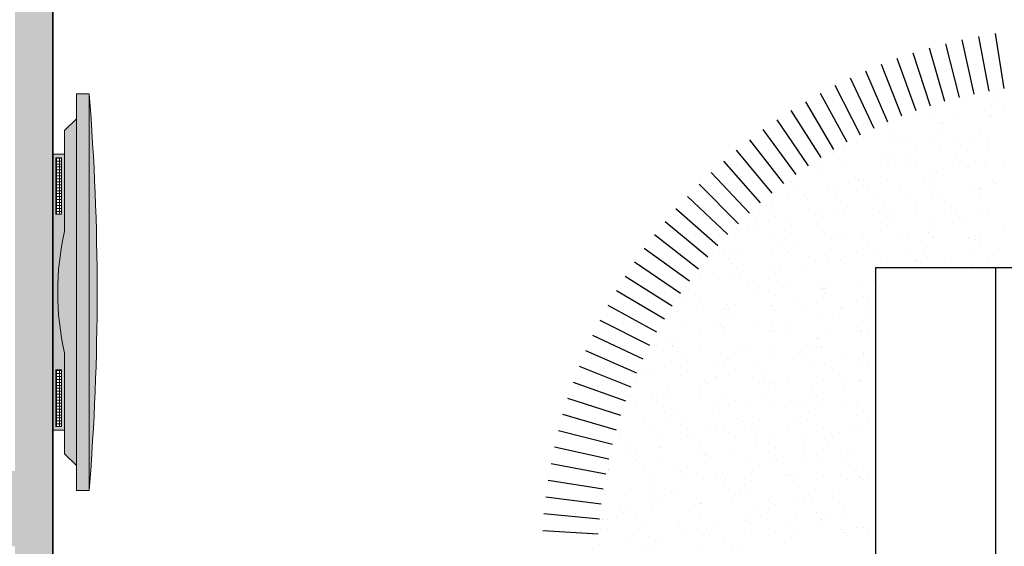
# Model space of a CAD drawing. Units: inches. Extents: x 1566 to 2546, y 1087 to 2705.
# Tile 4 of 27: x 1820 to 1925, y 1270 to 1326. Entities that reach past the tile are written whole.
import ezdxf

# ---------------------------------------------------------------- set-up
doc = ezdxf.new("R2010")
doc.units = ezdxf.units.IN
for name, color, linetype in [('A-FRN', 11, 'Continuous'), ('A-HT', 15, 'Continuous'), ('L-HT', 1, 'Continuous')]:
    doc.layers.add(name, color=color, linetype=linetype)
for name, color, linetype, lineweight in [('A-FURN', 8, 'Continuous', 18), ('A-WALL', 7, 'Continuous', 35), ('A-WALL-PATT', 8, 'Continuous', 13), ('moveis', 254, 'Continuous', 5), ('parede', 7, 'Continuous', 30)]:
    doc.layers.add(name, color=color, linetype=linetype, lineweight=lineweight)

# ---------------------------------------------------------------- blocks, each defined once
blk = doc.blocks.new('*X21')
at = {"color": 0}
for p, q in [((1.945, 2.8452), (1.945, 2.8452)), ((1.7428, 2.8186), (1.7428, 2.8186)), ((1.7438, 2.8187), (1.7438, 2.8187)), ((1.7537, 2.8227), (1.7537, 2.8227)), ((1.7698, 2.8221), (1.7698, 2.8221)), ((1.8017, 2.833), (1.8017, 2.833)), ((1.8104, 2.8275), (1.8104, 2.8275)), ((1.8778, 2.8235), (1.8778, 2.8235)), ((1.8783, 2.8364), (1.8783, 2.8364)), ((1.9044, 2.8399), (1.9044, 2.8399)), ((1.9094, 2.823), (1.9094, 2.823)), ((1.6514, 2.7891), (1.6514, 2.7891)), ((1.8515, 2.7874), (1.8515, 2.7874)), ((1.5474, 2.7675), (1.5474, 2.7675)), ((1.6825, 2.7724), (1.6825, 2.7724)), ((1.8133, 2.774), (1.8133, 2.774)), ((1.8607, 2.779), (1.8607, 2.779)), ((1.9412, 2.7734), (1.9412, 2.7734)), ((1.5011, 2.7453), (1.5011, 2.7453)), ((1.5414, 2.759), (1.5414, 2.759)), ((1.5625, 2.7456), (1.5625, 2.7456)), ((1.6971, 2.7593), (1.6971, 2.7593)), ((1.7012, 2.7435), (1.7012, 2.7435)), ((1.7104, 2.7351), (1.7104, 2.7351)), ((1.7182, 2.7459), (1.7182, 2.7459)), ((1.8528, 2.7596), (1.8528, 2.7596)), ((1.8739, 2.7462), (1.8739, 2.7462)), ((1.9042, 2.7391), (1.9042, 2.7391)), ((1.4871, 2.7212), (1.4871, 2.7212)), ((1.618, 2.7229), (1.618, 2.7229)), ((1.7459, 2.7223), (1.7459, 2.7223)), ((1.881, 2.7272), (1.881, 2.7272)), ((1.9244, 2.7131), (1.9244, 2.7131)), ((1.9505, 2.7165), (1.9505, 2.7165)), ((1.4827, 2.697), (1.4827, 2.697)), ((1.5509, 2.6997), (1.5509, 2.6997)), ((1.5601, 2.6912), (1.5601, 2.6912)), ((1.6384, 2.6973), (1.6384, 2.6973)), ((1.6813, 2.681), (1.6813, 2.681)), ((1.7219, 2.6864), (1.7219, 2.6864)), ((1.7539, 2.6952), (1.7539, 2.6952)), ((1.7899, 2.6953), (1.7899, 2.6953)), ((1.7941, 2.6975), (1.7941, 2.6975)), ((1.8159, 2.6988), (1.8159, 2.6988)), ((1.8565, 2.7041), (1.8565, 2.7041)), ((1.9498, 2.6978), (1.9498, 2.6978)), ((1.4006, 2.6558), (1.4006, 2.6558)), ((1.4227, 2.6718), (1.4227, 2.6718)), ((1.5207, 2.6599), (1.5207, 2.6599)), ((1.5467, 2.6633), (1.5467, 2.6633)), ((1.5506, 2.6712), (1.5506, 2.6712)), ((1.5873, 2.6687), (1.5873, 2.6687)), ((1.6553, 2.6776), (1.6553, 2.6776)), ((1.6856, 2.676), (1.6856, 2.676)), ((1.8165, 2.6777), (1.8165, 2.6777)), ((1.9444, 2.6771), (1.9444, 2.6771)), ((1.2775, 2.6279), (1.2775, 2.6279)), ((1.3182, 2.6332), (1.3182, 2.6332)), ((1.3861, 2.6422), (1.3861, 2.6422)), ((1.4098, 2.6473), (1.4098, 2.6473)), ((1.4121, 2.6456), (1.4121, 2.6456)), ((1.4261, 2.6336), (1.4261, 2.6336)), ((1.4528, 2.651), (1.4528, 2.651)), ((1.5818, 2.6338), (1.5818, 2.6338)), ((1.6036, 2.6513), (1.6036, 2.6513)), ((1.7375, 2.6341), (1.7375, 2.6341)), ((1.8037, 2.6496), (1.8037, 2.6496)), ((1.8129, 2.6412), (1.8129, 2.6412)), ((1.8841, 2.6308), (1.8841, 2.6308)), ((1.8932, 2.6344), (1.8932, 2.6344)), ((1.2503, 2.6119), (1.2503, 2.6119)), ((1.2595, 2.6034), (1.2595, 2.6034)), ((1.2915, 2.6198), (1.2915, 2.6198)), ((1.3552, 2.62), (1.3552, 2.62)), ((1.4472, 2.6201), (1.4472, 2.6201)), ((1.4533, 2.6075), (1.4533, 2.6075)), ((1.4903, 2.6249), (1.4903, 2.6249)), ((1.6029, 2.6204), (1.6029, 2.6204)), ((1.6212, 2.6266), (1.6212, 2.6266)), ((1.6534, 2.6057), (1.6534, 2.6057)), ((1.7491, 2.626), (1.7491, 2.626)), ((1.7586, 2.6207), (1.7586, 2.6207)), ((1.8564, 2.6013), (1.8564, 2.6013)), ((1.9143, 2.621), (1.9143, 2.621)), ((1.4258, 2.5754), (1.4258, 2.5754)), ((1.5537, 2.5748), (1.5537, 2.5748)), ((1.6626, 2.5973), (1.6626, 2.5973)), ((1.6888, 2.5797), (1.6888, 2.5797)), ((1.8196, 2.5814), (1.8196, 2.5814)), ((1.862, 2.5754), (1.862, 2.5754)), ((1.9026, 2.5807), (1.9026, 2.5807)), ((1.9475, 2.5807), (1.9475, 2.5807)), ((1.2117, 2.5712), (1.2117, 2.5712)), ((1.2949, 2.5738), (1.2949, 2.5738)), ((1.303, 2.5636), (1.303, 2.5636)), ((1.3674, 2.5715), (1.3674, 2.5715)), ((1.5031, 2.5619), (1.5031, 2.5619)), ((1.5123, 2.5534), (1.5123, 2.5534)), ((1.5231, 2.5718), (1.5231, 2.5718)), ((1.6788, 2.572), (1.6788, 2.572)), ((1.7014, 2.5542), (1.7014, 2.5542)), ((1.7061, 2.5574), (1.7061, 2.5574)), ((1.7274, 2.5577), (1.7274, 2.5577)), ((1.768, 2.563), (1.768, 2.563)), ((1.8345, 2.5723), (1.8345, 2.5723)), ((1.836, 2.5719), (1.836, 2.5719)), ((1.9061, 2.5557), (1.9061, 2.5557)), ((1.2305, 2.5243), (1.2305, 2.5243)), ((1.3584, 2.5237), (1.3584, 2.5237)), ((1.4582, 2.5222), (1.4582, 2.5222)), ((1.4934, 2.5286), (1.4934, 2.5286)), ((1.4989, 2.5276), (1.4989, 2.5276)), ((1.5668, 2.5365), (1.5668, 2.5365)), ((1.5928, 2.5399), (1.5928, 2.5399)), ((1.6243, 2.5302), (1.6243, 2.5302)), ((1.6334, 2.5453), (1.6334, 2.5453)), ((1.7522, 2.5296), (1.7522, 2.5296)), ((1.8873, 2.5345), (1.8873, 2.5345)), ((1.9154, 2.5473), (1.9154, 2.5473)), ((1.1527, 2.5197), (1.1527, 2.5197)), ((1.1551, 2.5078), (1.1551, 2.5078)), ((1.2976, 2.5011), (1.2976, 2.5011)), ((1.3108, 2.5081), (1.3108, 2.5081)), ((1.3236, 2.5045), (1.3236, 2.5045)), ((1.3527, 2.518), (1.3527, 2.518)), ((1.362, 2.5095), (1.362, 2.5095)), ((1.3643, 2.5098), (1.3643, 2.5098)), ((1.4322, 2.5188), (1.4322, 2.5188)), ((1.4665, 2.5083), (1.4665, 2.5083)), ((1.5558, 2.5136), (1.5558, 2.5136)), ((1.6222, 2.5086), (1.6222, 2.5086)), ((1.6433, 2.4952), (1.6433, 2.4952)), ((1.7558, 2.5118), (1.7558, 2.5118)), ((1.7651, 2.5034), (1.7651, 2.5034)), ((1.7779, 2.5089), (1.7779, 2.5089)), ((1.799, 2.4955), (1.799, 2.4955)), ((1.9336, 2.5092), (1.9336, 2.5092)), ((1.0951, 2.4744), (1.0951, 2.4744)), ((1.163, 2.4833), (1.163, 2.4833)), ((1.163, 2.4726), (1.163, 2.4726)), ((1.1761, 2.4943), (1.1761, 2.4943)), ((1.189, 2.4868), (1.189, 2.4868)), ((1.2024, 2.4741), (1.2024, 2.4741)), ((1.2297, 2.4921), (1.2297, 2.4921)), ((1.2981, 2.4774), (1.2981, 2.4774)), ((1.3319, 2.4946), (1.3319, 2.4946)), ((1.4055, 2.4697), (1.4055, 2.4697)), ((1.429, 2.4791), (1.429, 2.4791)), ((1.4876, 2.4949), (1.4876, 2.4949)), ((1.5569, 2.4785), (1.5569, 2.4785)), ((1.6919, 2.4833), (1.6919, 2.4833)), ((1.8228, 2.485), (1.8228, 2.485)), ((1.9507, 2.4844), (1.9507, 2.4844)), ((1.0963, 2.4457), (1.0963, 2.4457)), ((1.2117, 2.4657), (1.2117, 2.4657)), ((1.2521, 2.446), (1.2521, 2.446)), ((1.4078, 2.4463), (1.4078, 2.4463)), ((1.5635, 2.4466), (1.5635, 2.4466)), ((1.6055, 2.468), (1.6055, 2.468)), ((1.6148, 2.4595), (1.6148, 2.4595)), ((1.7192, 2.4468), (1.7192, 2.4468)), ((1.8086, 2.4635), (1.8086, 2.4635)), ((1.8749, 2.4471), (1.8749, 2.4471)), ((1.8821, 2.4486), (1.8821, 2.4486)), ((1.9081, 2.452), (1.9081, 2.452)), ((1.9487, 2.4573), (1.9487, 2.4573)), ((1.0521, 2.4302), (1.0521, 2.4302)), ((1.0613, 2.4218), (1.0613, 2.4218)), ((1.1027, 2.4263), (1.1027, 2.4263)), ((1.2336, 2.428), (1.2336, 2.428)), ((1.2552, 2.4258), (1.2552, 2.4258)), ((1.3615, 2.4273), (1.3615, 2.4273)), ((1.4552, 2.4241), (1.4552, 2.4241)), ((1.4644, 2.4156), (1.4644, 2.4156)), ((1.4966, 2.4322), (1.4966, 2.4322)), ((1.6275, 2.4339), (1.6275, 2.4339)), ((1.6389, 2.4165), (1.6389, 2.4165)), ((1.6582, 2.4197), (1.6582, 2.4197)), ((1.6795, 2.4219), (1.6795, 2.4219)), ((1.7475, 2.4308), (1.7475, 2.4308)), ((1.7554, 2.4333), (1.7554, 2.4333)), ((1.7735, 2.4343), (1.7735, 2.4343)), ((1.8141, 2.4396), (1.8141, 2.4396)), ((1.8583, 2.4179), (1.8583, 2.4179)), ((1.8904, 2.4381), (1.8904, 2.4381)), ((1.4783, 2.3954), (1.4783, 2.3954)), ((1.5043, 2.3988), (1.5043, 2.3988)), ((1.545, 2.4042), (1.545, 2.4042)), ((1.6129, 2.4131), (1.6129, 2.4131)), ((1.8675, 2.4095), (1.8675, 2.4095)), ((1.0383, 2.3768), (1.0383, 2.3768)), ((1.0397, 2.3823), (1.0397, 2.3823)), ((1.0608, 2.3689), (1.0608, 2.3689)), ((1.1048, 2.3819), (1.1048, 2.3819)), ((1.1662, 2.3762), (1.1662, 2.3762)), ((1.1954, 2.3826), (1.1954, 2.3826)), ((1.2165, 2.3691), (1.2165, 2.3691)), ((1.2351, 2.3634), (1.2351, 2.3634)), ((1.2758, 2.3687), (1.2758, 2.3687)), ((1.3012, 2.3811), (1.3012, 2.3811)), ((1.3049, 2.3802), (1.3049, 2.3802)), ((1.3141, 2.3717), (1.3141, 2.3717)), ((1.3437, 2.3777), (1.3437, 2.3777)), ((1.3512, 2.3829), (1.3512, 2.3829)), ((1.3697, 2.3811), (1.3697, 2.3811)), ((1.3722, 2.3694), (1.3722, 2.3694)), ((1.4104, 2.3865), (1.4104, 2.3865)), ((1.4321, 2.3828), (1.4321, 2.3828)), ((1.5069, 2.3831), (1.5069, 2.3831)), ((1.5079, 2.3758), (1.5079, 2.3758)), ((1.5279, 2.3697), (1.5279, 2.3697)), ((1.56, 2.3821), (1.56, 2.3821)), ((1.6626, 2.3834), (1.6626, 2.3834)), ((1.6837, 2.37), (1.6837, 2.37)), ((1.6951, 2.387), (1.6951, 2.387)), ((1.708, 2.374), (1.708, 2.374)), ((1.7172, 2.3656), (1.7172, 2.3656)), ((1.8183, 2.3837), (1.8183, 2.3837)), ((1.8259, 2.3887), (1.8259, 2.3887)), ((1.8394, 2.3703), (1.8394, 2.3703)), ((1.911, 2.3696), (1.911, 2.3696)), ((1.0745, 2.3422), (1.0745, 2.3422)), ((1.1005, 2.3457), (1.1005, 2.3457)), ((1.1412, 2.351), (1.1412, 2.351)), ((1.1546, 2.3363), (1.1546, 2.3363)), ((1.2091, 2.36), (1.2091, 2.36)), ((1.4997, 2.3359), (1.4997, 2.3359)), ((1.6306, 2.3375), (1.6306, 2.3375)), ((1.7585, 2.3369), (1.7585, 2.3369)), ((1.8936, 2.3418), (1.8936, 2.3418)), ((0.966, 2.3279), (0.966, 2.3279)), ((0.9708, 2.3251), (0.9708, 2.3251)), ((0.981, 2.3202), (0.981, 2.3202)), ((1.0066, 2.3333), (1.0066, 2.3333)), ((1.1059, 2.33), (1.1059, 2.33)), ((1.1367, 2.3205), (1.1367, 2.3205)), ((1.1638, 2.3279), (1.1638, 2.3279)), ((1.2368, 2.3316), (1.2368, 2.3316)), ((1.2924, 2.3208), (1.2924, 2.3208)), ((1.3576, 2.3319), (1.3576, 2.3319)), ((1.3647, 2.331), (1.3647, 2.331)), ((1.4481, 2.3211), (1.4481, 2.3211)), ((1.5577, 2.3302), (1.5577, 2.3302)), ((1.5669, 2.3217), (1.5669, 2.3217)), ((1.6038, 2.3214), (1.6038, 2.3214)), ((1.7596, 2.3216), (1.7596, 2.3216)), ((1.7607, 2.3257), (1.7607, 2.3257)), ((1.8196, 2.3109), (1.8196, 2.3109)), ((1.8602, 2.3162), (1.8602, 2.3162)), ((1.9153, 2.3219), (1.9153, 2.3219)), ((1.9282, 2.3252), (1.9282, 2.3252)), ((1.0043, 2.2924), (1.0043, 2.2924)), ((1.0135, 2.284), (1.0135, 2.284)), ((1.2073, 2.288), (1.2073, 2.288)), ((1.3044, 2.2847), (1.3044, 2.2847)), ((1.4074, 2.2863), (1.4074, 2.2863)), ((1.4353, 2.2864), (1.4353, 2.2864)), ((1.5632, 2.2858), (1.5632, 2.2858)), ((1.659, 2.2897), (1.659, 2.2897)), ((1.685, 2.2932), (1.685, 2.2932)), ((1.6982, 2.2907), (1.6982, 2.2907)), ((1.7256, 2.2985), (1.7256, 2.2985)), ((1.7936, 2.3074), (1.7936, 2.3074)), ((1.8291, 2.2923), (1.8291, 2.2923)), ((0.9244, 2.2568), (0.9244, 2.2568)), ((1.0414, 2.2805), (1.0414, 2.2805)), ((1.0801, 2.2571), (1.0801, 2.2571)), ((1.1693, 2.2799), (1.1693, 2.2799)), ((1.2358, 2.2574), (1.2358, 2.2574)), ((1.3915, 2.2577), (1.3915, 2.2577)), ((1.4158, 2.2577), (1.4158, 2.2577)), ((1.4166, 2.2778), (1.4166, 2.2778)), ((1.4565, 2.2631), (1.4565, 2.2631)), ((1.5244, 2.272), (1.5244, 2.272)), ((1.5472, 2.2579), (1.5472, 2.2579)), ((1.5504, 2.2754), (1.5504, 2.2754)), ((1.5911, 2.2808), (1.5911, 2.2808)), ((1.6104, 2.2819), (1.6104, 2.2819)), ((1.7029, 2.2582), (1.7029, 2.2582)), ((1.8105, 2.2801), (1.8105, 2.2801)), ((1.8197, 2.2717), (1.8197, 2.2717)), ((1.8587, 2.2585), (1.8587, 2.2585)), ((0.9455, 2.2434), (0.9455, 2.2434)), ((1.057, 2.2441), (1.057, 2.2441)), ((1.1012, 2.2437), (1.1012, 2.2437)), ((1.109, 2.2336), (1.109, 2.2336)), ((1.2399, 2.2353), (1.2399, 2.2353)), ((1.2552, 2.2366), (1.2552, 2.2366)), ((1.2569, 2.2439), (1.2569, 2.2439)), ((1.2571, 2.2424), (1.2571, 2.2424)), ((1.2663, 2.234), (1.2663, 2.234)), ((1.2812, 2.24), (1.2812, 2.24)), ((1.3219, 2.2453), (1.3219, 2.2453)), ((1.3678, 2.2347), (1.3678, 2.2347)), ((1.3898, 2.2543), (1.3898, 2.2543)), ((1.4126, 2.2442), (1.4126, 2.2442)), ((1.4601, 2.238), (1.4601, 2.238)), ((1.5029, 2.2395), (1.5029, 2.2395)), ((1.5683, 2.2445), (1.5683, 2.2445)), ((1.6338, 2.2412), (1.6338, 2.2412)), ((1.6602, 2.2363), (1.6602, 2.2363)), ((1.724, 2.2448), (1.724, 2.2448)), ((1.7617, 2.2406), (1.7617, 2.2406)), ((1.8632, 2.2318), (1.8632, 2.2318)), ((1.8797, 2.2451), (1.8797, 2.2451)), ((1.8967, 2.2455), (1.8967, 2.2455)), ((0.974, 2.2287), (0.974, 2.2287)), ((1.0121, 2.2046), (1.0121, 2.2046)), ((1.0527, 2.2099), (1.0527, 2.2099)), ((1.1206, 2.2189), (1.1206, 2.2189)), ((1.1466, 2.2223), (1.1466, 2.2223)), ((1.1873, 2.2276), (1.1873, 2.2276)), ((1.6694, 2.2278), (1.6694, 2.2278)), ((0.8775, 2.1868), (0.8775, 2.1868)), ((0.9067, 2.2002), (0.9067, 2.2002)), ((0.9137, 2.1825), (0.9137, 2.1825)), ((0.9181, 2.1922), (0.9181, 2.1922)), ((0.986, 2.2011), (0.986, 2.2011)), ((1.0214, 2.195), (1.0214, 2.195)), ((1.0446, 2.1841), (1.0446, 2.1841)), ((1.1068, 2.1985), (1.1068, 2.1985)), ((1.116, 2.1901), (1.116, 2.1901)), ((1.1725, 2.1835), (1.1725, 2.1835)), ((1.1771, 2.1953), (1.1771, 2.1953)), ((1.3075, 2.1884), (1.3075, 2.1884)), ((1.3098, 2.1941), (1.3098, 2.1941)), ((1.3328, 2.1956), (1.3328, 2.1956)), ((1.4384, 2.1901), (1.4384, 2.1901)), ((1.4885, 2.1959), (1.4885, 2.1959)), ((1.5099, 2.1924), (1.5099, 2.1924)), ((1.5191, 2.1839), (1.5191, 2.1839)), ((1.5663, 2.1895), (1.5663, 2.1895)), ((1.6442, 2.1961), (1.6442, 2.1961)), ((1.7014, 2.1943), (1.7014, 2.1943)), ((1.7129, 2.188), (1.7129, 2.188)), ((1.7999, 2.1964), (1.7999, 2.1964)), ((1.8322, 2.196), (1.8322, 2.196)), ((1.8397, 2.1841), (1.8397, 2.1841)), ((1.8657, 2.1875), (1.8657, 2.1875)), ((1.9063, 2.1928), (1.9063, 2.1928)), ((1.913, 2.1862), (1.913, 2.1862)), ((1.9222, 2.1778), (1.9222, 2.1778)), ((0.9565, 2.1546), (0.9565, 2.1546)), ((1.1595, 2.1502), (1.1595, 2.1502)), ((1.5965, 2.152), (1.5965, 2.152)), ((1.6372, 2.1574), (1.6372, 2.1574)), ((1.7051, 2.1663), (1.7051, 2.1663)), ((1.7311, 2.1698), (1.7311, 2.1698)), ((1.7717, 2.1751), (1.7717, 2.1751)), ((0.8492, 2.133), (0.8492, 2.133)), ((0.9648, 2.1316), (0.9648, 2.1316)), ((0.9657, 2.1462), (0.9657, 2.1462)), ((0.9771, 2.1324), (0.9771, 2.1324)), ((1.1122, 2.1373), (1.1122, 2.1373)), ((1.1205, 2.1319), (1.1205, 2.1319)), ((1.2431, 2.1389), (1.2431, 2.1389)), ((1.2762, 2.1322), (1.2762, 2.1322)), ((1.3596, 2.1485), (1.3596, 2.1485)), ((1.3688, 2.14), (1.3688, 2.14)), ((1.371, 2.1383), (1.371, 2.1383)), ((1.4319, 2.1324), (1.4319, 2.1324)), ((1.4359, 2.1309), (1.4359, 2.1309)), ((1.4619, 2.1343), (1.4619, 2.1343)), ((1.5026, 2.1397), (1.5026, 2.1397)), ((1.506, 2.1432), (1.506, 2.1432)), ((1.5626, 2.1441), (1.5626, 2.1441)), ((1.5705, 2.1486), (1.5705, 2.1486)), ((1.5876, 2.1327), (1.5876, 2.1327)), ((1.6369, 2.1449), (1.6369, 2.1449)), ((1.7433, 2.133), (1.7433, 2.133)), ((1.7627, 2.1424), (1.7627, 2.1424)), ((1.7648, 2.1442), (1.7648, 2.1442)), ((1.7719, 2.1339), (1.7719, 2.1339)), ((1.899, 2.1333), (1.899, 2.1333)), ((1.8999, 2.1491), (1.8999, 2.1491)), ((0.9859, 2.1182), (0.9859, 2.1182)), ((1.0092, 2.1063), (1.0092, 2.1063)), ((1.1416, 2.1184), (1.1416, 2.1184)), ((1.1927, 2.0989), (1.1927, 2.0989)), ((1.2093, 2.1046), (1.2093, 2.1046)), ((1.2334, 2.1042), (1.2334, 2.1042)), ((1.2973, 2.1187), (1.2973, 2.1187)), ((1.3013, 2.1132), (1.3013, 2.1132)), ((1.3273, 2.1166), (1.3273, 2.1166)), ((1.368, 2.122), (1.368, 2.122)), ((1.4123, 2.1002), (1.4123, 2.1002)), ((1.453, 2.119), (1.453, 2.119)), ((1.6087, 2.1193), (1.6087, 2.1193)), ((1.7644, 2.1196), (1.7644, 2.1196)), ((1.9201, 2.1199), (1.9201, 2.1199)), ((0.9169, 2.0861), (0.9169, 2.0861)), ((1.0321, 2.0777), (1.0321, 2.0777)), ((1.0477, 2.0878), (1.0477, 2.0878)), ((1.0582, 2.0812), (1.0582, 2.0812)), ((1.0988, 2.0865), (1.0988, 2.0865)), ((1.1667, 2.0955), (1.1667, 2.0955)), ((1.1756, 2.0872), (1.1756, 2.0872)), ((0.8296, 2.0511), (0.8296, 2.0511)), ((0.8589, 2.0624), (0.8589, 2.0624)), ((0.8975, 2.06), (0.8975, 2.06)), ((0.9061, 2.0695), (0.9061, 2.0695)), ((0.9236, 2.0635), (0.9236, 2.0635)), ((0.9642, 2.0688), (0.9642, 2.0688)), ((1.059, 2.0607), (1.059, 2.0607)), ((1.0618, 2.0698), (1.0618, 2.0698)), ((1.0682, 2.0523), (1.0682, 2.0523)), ((0.8524, 2.0367), (0.8524, 2.0367)), ((0.9803, 2.0361), (0.9803, 2.0361)), ((1.1153, 2.0409), (1.1153, 2.0409)), ((0.8495, 2.0061), (0.8495, 2.0061)), ((0.8706, 1.9927), (0.8706, 1.9927)), ((0.9087, 2.0168), (0.9087, 2.0168)), ((0.9179, 2.0084), (0.9179, 2.0084)), ((1.0052, 2.0064), (1.0052, 2.0064)), ((1.0263, 1.993), (1.0263, 1.993)), ((1.0509, 1.9915), (1.0509, 1.9915)), ((1.1117, 2.0124), (1.1117, 2.0124)), ((1.1609, 2.0067), (1.1609, 2.0067)), ((1.1788, 1.9909), (1.1788, 1.9909)), ((1.182, 1.9932), (1.182, 1.9932)), ((0.785, 1.9849), (0.785, 1.9849)), ((0.92, 1.9898), (0.92, 1.9898)), ((0.9614, 1.9685), (0.9614, 1.9685)), ((1.1614, 1.9668), (1.1614, 1.9668)), ((0.7908, 1.944), (0.7908, 1.944)), ((0.8555, 1.9403), (0.8555, 1.9403)), ((0.9465, 1.9443), (0.9465, 1.9443)), ((0.9697, 1.9401), (0.9697, 1.9401)), ((0.9834, 1.9397), (0.9834, 1.9397)), ((1.0103, 1.9454), (1.0103, 1.9454)), ((1.0782, 1.9544), (1.0782, 1.9544)), ((1.1022, 1.9446), (1.1022, 1.9446)), ((1.1043, 1.9578), (1.1043, 1.9578)), ((1.1185, 1.9446), (1.1185, 1.9446)), ((1.1449, 1.9631), (1.1449, 1.9631)), ((1.1707, 1.9584), (1.1707, 1.9584)), ((0.8091, 1.9189), (0.8091, 1.9189)), ((0.8111, 1.9247), (0.8111, 1.9247)), ((0.8351, 1.9223), (0.8351, 1.9223)), ((0.8757, 1.9277), (0.8757, 1.9277)), ((0.9436, 1.9366), (0.9436, 1.9366)), ((1.0111, 1.9229), (1.0111, 1.9229)), ((1.0204, 1.9145), (1.0204, 1.9145)), ((0.7881, 1.8886), (0.7881, 1.8886)), ((0.9232, 1.8935), (0.9232, 1.8935)), ((1.054, 1.8951), (1.054, 1.8951)), ((1.1819, 1.8945), (1.1819, 1.8945)), ((0.7552, 1.8672), (0.7552, 1.8672)), ((0.8608, 1.879), (0.8608, 1.879)), ((0.8701, 1.8706), (0.8701, 1.8706)), ((0.8898, 1.8809), (0.8898, 1.8809)), ((0.9109, 1.8675), (0.9109, 1.8675)), ((1.0456, 1.8812), (1.0456, 1.8812)), ((1.0639, 1.8746), (1.0639, 1.8746)), ((1.0666, 1.8678), (1.0666, 1.8678)), ((0.8587, 1.844), (0.8587, 1.844)), ((0.9866, 1.8434), (0.9866, 1.8434)), ((1.1216, 1.8482), (1.1216, 1.8482)), ((1.1504, 1.8344), (1.1504, 1.8344)), ((1.191, 1.8397), (1.191, 1.8397)), ((0.8311, 1.8188), (0.8311, 1.8188)), ((0.9136, 1.8307), (0.9136, 1.8307)), ((0.9868, 1.8191), (0.9868, 1.8191)), ((0.9897, 1.8132), (0.9897, 1.8132)), ((1.0158, 1.8167), (1.0158, 1.8167)), ((1.0564, 1.822), (1.0564, 1.822)), ((1.1136, 1.829), (1.1136, 1.829)), ((1.1228, 1.8206), (1.1228, 1.8206)), ((1.1243, 1.831), (1.1243, 1.831)), ((1.1425, 1.8194), (1.1425, 1.8194)), ((0.7466, 1.7812), (0.7466, 1.7812)), ((0.7632, 1.7869), (0.7632, 1.7869)), ((0.7872, 1.7866), (0.7872, 1.7866)), ((0.7913, 1.7922), (0.7913, 1.7922)), ((0.8552, 1.7955), (0.8552, 1.7955)), ((0.8812, 1.799), (0.8812, 1.799)), ((0.9218, 1.8043), (0.9218, 1.8043)), ((0.9263, 1.7971), (0.9263, 1.7971)), ((0.9633, 1.7851), (0.9633, 1.7851)), ((1.0572, 1.7988), (1.0572, 1.7988)), ((1.1663, 1.7807), (1.1663, 1.7807)), ((1.1851, 1.7982), (1.1851, 1.7982)), ((0.7206, 1.7778), (0.7206, 1.7778)), ((0.7745, 1.7554), (0.7745, 1.7554)), ((0.9302, 1.7557), (0.9302, 1.7557)), ((0.9725, 1.7767), (0.9725, 1.7767)), ((1.0859, 1.756), (1.0859, 1.756))]:
    blk.add_line(p, q, dxfattribs=at)
blk = doc.blocks.new('A$C6796526C')
at = {"layer": 'A-FRN'}
blk.add_lwpolyline([(0.65, 2.8), (0.65, 0.9), (2.25, 0.9), (2.25, 2.8)], dxfattribs=at)
at = {"layer": 'A-HT'}
for p, q in [((0.166, 1.2466), (0.0179, 1.2232)), ((0.173, 1.2064), (0.0257, 1.1783)), ((0.1813, 1.1664), (0.0349, 1.1337)), ((0.1908, 1.1267), (0.0456, 1.0894)), ((0.2016, 1.0873), (0.0576, 1.0455)), ((0.2136, 1.0483), (0.071, 1.0019)), ((0.2269, 1.0096), (0.0857, 0.9588)), ((0.2413, 0.9714), (0.1018, 0.9162)), ((0.2569, 0.9337), (0.1193, 0.8741)), ((0.2737, 0.8965), (0.138, 0.8326)), ((0.2917, 0.8598), (0.158, 0.7917)), ((0.3108, 0.8237), (0.1794, 0.7515)), ((0.331, 0.7882), (0.2019, 0.7119)), ((0.3524, 0.7534), (0.2257, 0.6731)), ((0.3748, 0.7193), (0.2507, 0.635)), ((0.3983, 0.6859), (0.2769, 0.5977)), ((0.4228, 0.6532), (0.3043, 0.5613)), ((0.4483, 0.6213), (0.3328, 0.5257)), ((0.4749, 0.5903), (0.3623, 0.4911)), ((0.5023, 0.5601), (0.393, 0.4574)), ((0.5308, 0.5308), (0.4247, 0.4247)), ((0.5601, 0.5023), (0.4574, 0.393)), ((0.5903, 0.4749), (0.4911, 0.3623)), ((0.6213, 0.4483), (0.5257, 0.3328)), ((0.6532, 0.4228), (0.5613, 0.3043)), ((0.6859, 0.3983), (0.5977, 0.2769)), ((0.7193, 0.3748), (0.635, 0.2507)), ((0.7534, 0.3524), (0.6731, 0.2257)), ((0.7882, 0.331), (0.7119, 0.2019)), ((0.8237, 0.3108), (0.7515, 0.1794)), ((0.8598, 0.2917), (0.7917, 0.158)), ((0.8965, 0.2737), (0.8326, 0.138)), ((0.9337, 0.2569), (0.8741, 0.1193)), ((0.9714, 0.2413), (0.9162, 0.1018)), ((1.0096, 0.2269), (0.9588, 0.0857)), ((1.0483, 0.2136), (1.0019, 0.071)), ((1.0873, 0.2016), (1.0455, 0.0576)), ((1.1267, 0.1908), (1.0894, 0.0456)), ((1.1664, 0.1813), (1.1337, 0.0349)), ((1.2064, 0.173), (1.1783, 0.0257)), ((1.2466, 0.166), (1.2232, 0.0179)), ((1.2871, 0.1603), (1.2683, 0.0114)), ((1.3277, 0.1558), (1.3135, 0.0064)), ((1.3684, 0.1526), (1.359, 0.0029))]:
    blk.add_line(p, q, dxfattribs=at)
at = {"layer": 'L-HT'}
blk.add_line((1.7809, 1.2249), (0.65, 1.2249), dxfattribs=at)
at = {"layer": 'A-HT', "extrusion": (0, 0, -1), "zscale": -1, "rotation": 180}
blk.add_blockref('*X21', (0.55, 3), dxfattribs=at)
blk = doc.blocks.new('PLASMA 2')
at = {"layer": 'moveis', "ltscale": 0.08}
h = blk.add_hatch(dxfattribs=at)
h.set_pattern_fill('_USER,_O', color=256, scale=0.008, double=1, pattern_type=0)
h.set_pattern_definition([(360, (-4.134502, -6.848382), (0, 0.008), []), (90, (-4.134502, -6.848382), (-0.008, 0), [])])
h.paths.add_polyline_path([(-0.2099, -0.0965), (-0.3623, -0.0965), (-0.3623, -0.1111), (-0.2099, -0.1111)])
h = blk.add_hatch(dxfattribs=at)
h.set_pattern_fill('_USER,_O', color=256, scale=0.008, double=1, pattern_type=0)
h.set_pattern_definition([(180, (4.134502, -6.848382), (0, 0.008), []), (90, (4.134502, -6.848382), (0.008, 0), [])])
h.paths.add_polyline_path([(0.2099, -0.0965), (0.3623, -0.0965), (0.3623, -0.1111), (0.2099, -0.1111)])
at = {"layer": 'parede', "ltscale": 0.08}
h = blk.add_hatch(color=256, dxfattribs=at)
h.dxf.hatch_style = 1
h.set_gradient(color1=(131, 136, 145), one_color=1, tint=1, name='CURVED')
h.paths.add_polyline_path([(-0.535, -0.0215), (0.535, -0.0215, 0.040195)])
h = blk.add_hatch(color=256, dxfattribs=at)
h.dxf.hatch_style = 1
h.set_gradient(color1=(131, 136, 145), color2=(0, 0, 0), one_color=1, name='CURVED')
h.paths.add_polyline_path([(0.535, -0.0215), (-0.535, -0.0215), (-0.535, -0.0553), (0.535, -0.0553)])
h = blk.add_hatch(color=256, dxfattribs=at)
h.dxf.hatch_style = 1
h.set_gradient(color1=(131, 136, 145), one_color=1, tint=1, name='CYLINDER')
h.paths.add_polyline_path([(0.4673, -0.0553), (-0.4673, -0.0553), (-0.4363, -0.0876), (-0.1636, -0.0876, 0.114423), (0.1636, -0.0876), (0.4363, -0.0876)])
h = blk.add_hatch(color=256, dxfattribs=at)
h.dxf.hatch_style = 1
h.set_gradient(color1=(131, 136, 145), color2=(0, 0, 0), one_color=1, name='CURVED')
h.paths.add_polyline_path([(0.3724, -0.0876), (0.1636, -0.0876, -0.114423), (-0.1636, -0.0876), (-0.3724, -0.0876), (-0.3724, -0.12), (0.3724, -0.12)])
h.paths.add_polyline_path([(-0.2099, -0.1111), (-0.3623, -0.1111), (-0.3623, -0.0965), (-0.2099, -0.0965)], flags=16)
h.paths.add_polyline_path([(0.2099, -0.1111), (0.2099, -0.0965), (0.3623, -0.0965), (0.3623, -0.1111)], flags=16)
at = {"layer": 'moveis', "ltscale": 0.08}
for p, q in [((-0.535, -0.0215), (-0.535, -0.0553)), ((-0.535, -0.0215), (0.535, -0.0215)), ((0.535, -0.0553), (0.535, -0.0215)), ((0.535, -0.0553), (-0.535, -0.0553)), ((-0.4673, -0.0553), (-0.4363, -0.0876)), ((0.4673, -0.0553), (0.4363, -0.0876)), ((-0.4363, -0.0876), (-0.1636, -0.0876)), ((-0.3724, -0.0876), (-0.3724, -0.12)), ((0.1636, -0.0876), (0.4363, -0.0876)), ((0.3724, -0.0876), (0.3724, -0.12)), ((-0.3724, -0.12), (0.3724, -0.12))]:
    blk.add_line(p, q, dxfattribs=at)
for points in [[(-0.3623, -0.0965), (-0.2099, -0.0965), (-0.2099, -0.1111), (-0.3623, -0.1111)], [(0.3623, -0.0965), (0.2099, -0.0965), (0.2099, -0.1111), (0.3623, -0.1111)]]:
    blk.add_lwpolyline(points, close=True, dxfattribs=at)
for centre, radius, start, end in [((0, -6.6658), 6.6658, 85.39647, 94.60353), ((0, 0.6178), 0.7242, 256.9449, 283.0551)]:
    blk.add_arc(centre, radius, start, end, dxfattribs=at)

msp = doc.modelspace()

# ---------------------------------------------------------------- hatches: boundary and pattern name
at = {"layer": 'A-WALL-PATT'}
h = msp.add_hatch(color=256, dxfattribs=at)
h.dxf.hatch_style = 1
h.paths.add_polyline_path([(2001.53, 1778.2), (1641.53, 1778.2), (1641.53, 1746.2), (1649.53, 1746.2), (1649.53, 1770.2), (1769.53, 1770.2), (1769.53, 1650.2), (1767.53, 1650.2), (1767.53, 1648.2), (1767.53, 1646.2), (1819.53, 1646.2), (1819.53, 1650.2), (1773.53, 1650.2), (1773.53, 1770.2), (1941.53, 1770.2), (1941.53, 1756.2), (1945.53, 1756.2), (1945.53, 1770.2), (1993.53, 1770.2), (1993.53, 1650.2), (1945.53, 1650.2), (1945.53, 1652.2), (1943.53, 1652.2), (1941.53, 1652.2), (1941.53, 1650.2), (1867.53, 1650.2), (1867.53, 1642.2), (1871.53, 1642.2), (1871.53, 1646.2), (1993.53, 1646.2), (1993.53, 1526.2), (1871.53, 1526.2), (1871.53, 1606.2), (1867.53, 1606.2), (1867.53, 1522.2), (1993.53, 1522.2), (1993.53, 1387.2), (1959.53, 1387.2), (1959.53, 1397.2), (1955.53, 1397.2), (1955.53, 1387.2), (1903.53, 1387.2), (1903.53, 1383.2), (1993.53, 1383.2), (1993.53, 1364.3), (1993.53, 1211.2), (1939.53, 1211.2), (1939.53, 1203.2), (1993.53, 1203.2), (1993.53, 1154.2), (2001.53, 1154.2)])
h.paths.add_polyline_path([(1649.53, 1646.2), (1731.53, 1646.2), (1731.53, 1650.2), (1649.53, 1650.2), (1649.53, 1674.2), (1641.53, 1674.2), (1641.53, 1622.2), (1649.53, 1622.2)], flags=17)
h.paths.add_polyline_path([(1649.53, 1550.2), (1641.53, 1550.2), (1641.53, 1510.2), (1649.53, 1510.2), (1649.53, 1522.2), (1731.53, 1522.2), (1731.53, 1500.2), (1735.53, 1500.2), (1735.53, 1522.2), (1767.53, 1522.2), (1767.53, 1500.2), (1771.53, 1500.2), (1771.53, 1526.2), (1649.53, 1526.2)], flags=17)
h.paths.add_polyline_path([(1649.53, 1464.2), (1735.53, 1464.2), (1735.53, 1470.2), (1731.53, 1470.2), (1731.53, 1468.2), (1649.53, 1468.2), (1649.53, 1480.2), (1641.53, 1480.2), (1641.53, 1419.2), (1649.53, 1419.2)], flags=17)
h.paths.add_polyline_path([(1649.53, 1323.2), (1641.53, 1323.2), (1641.53, 1270.2), (1667.53, 1270.2), (1667.53, 1278.2), (1649.53, 1278.2)], flags=17)
h.paths.add_polyline_path([(1763.53, 1278.2), (1727.53, 1278.2), (1727.53, 1270.2), (1763.53, 1270.2)], flags=17)
h.paths.add_polyline_path([(1823.53, 1383.2), (1827.53, 1383.2), (1827.53, 1385.2), (1827.53, 1387.2), (1819.53, 1387.2), (1819.53, 1324.21), (1819.53, 1278.2), (1811.53, 1278.2), (1811.53, 1274.2), (1811.53, 1270.2), (1819.53, 1270.2), (1819.53, 1203.2), (1877.53, 1203.2), (1877.53, 1211.2), (1823.53, 1211.2)], flags=17)

# ---------------------------------------------------------------- linework, layer by layer
at = {"layer": 'A-WALL'}
msp.add_line((1823.53, 1211.2), (1823.53, 1383.2), dxfattribs=at)

# ---------------------------------------------------------------- block references
at = {"layer": 'A-FURN', "xscale": 39.3701, "yscale": 39.3701, "zscale": 39.3701, "rotation": 270}
for name, p in [('A$C6796526C', (1875.42, 1325.37)), ('PLASMA 2', (1828.25, 1297.2))]:
    msp.add_blockref(name, p, dxfattribs=at)

doc.saveas('drawing.dxf')
